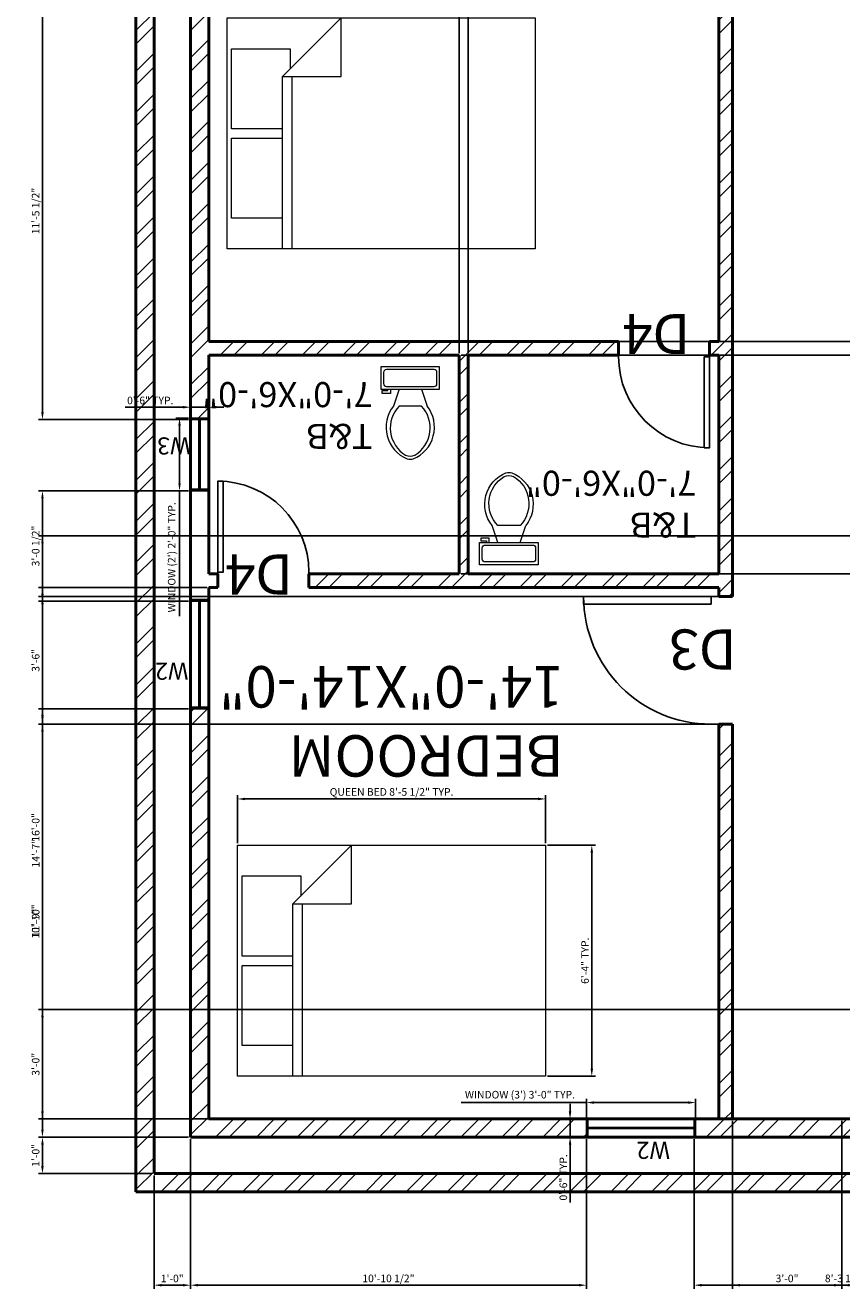
# Model space of a CAD drawing. Units: inches. Extents: x 244 to 2800, y 1060 to 1700.
# Tile 3 of 13: x 819 to 1088, y 1060 to 1477. Entities that reach past the tile are written whole.
import ezdxf

# ---------------------------------------------------------------- set-up
doc = ezdxf.new("R2010")
doc.units = ezdxf.units.IN
for name, color, linetype, lineweight in [('A-ANNO-DIMS', 2, 'Continuous', 18), ('A-ANNO-TEXT', 1, 'Continuous', 18), ('A-DOOR', 5, 'Continuous', 25), ('A-FURN', 9, 'Continuous', 18), ('A-GLAZ', 3, 'Continuous', 25), ('A-WALL', 7, 'Continuous', 50), ('A-WALL-PATT', 8, 'Continuous', 13)]:
    doc.layers.add(name, color=color, linetype=linetype, lineweight=lineweight)
doc.styles.get("Standard").update_dxf_attribs({"font": 'arial.ttf'})
doc.dimstyles.new('ISO-25', dxfattribs={"dimtxt": 2.5, "dimasz": 2.5, "dimexe": 1.25, "dimexo": 0.625, "dimtad": 1, "dimlunit": 4, "dimtxsty": 'Standard', "dimcen": 2.5, "dimadec": 0, "dimazin": 0, "dimtfac": 1, "dimtmove": 0, "dimatfit": 3, "dimfxl": 1, "dimarcsym": 0})

# ---------------------------------------------------------------- blocks, each defined once
blk = doc.blocks.new('*U2')
for p, q in [((0, 0), (0, -5)), ((30, 0), (30, -5))]:
    blk.add_line(p, q)
blk.add_lwpolyline([(0, 0), (0, 30), (1.75, 30), (1.75, 0)], close=True)
blk.add_arc((0, 0), 30, 0, 90)
blk = doc.blocks.new('Toilet - top')
for p, q in [((9.5, -6), (9.5, -2)), ((-10, -8.5), (-8, -8.5)), ((-10, -9.5), (-10, -8.5)), ((-8, -8.5), (-8, -8)), ((-7, -8), (-7, -9.5)), ((-4, -8), (-6, -14)), ((4, -8), (6, -14)), ((-7, -9.5), (-10, -9.5)), ((4, -14), (-4, -14))]:
    blk.add_line(p, q)
blk.add_lwpolyline([(10.5, -8), (10.5, 0), (-10.5, 0), (-10.5, -8)], close=True)
for points in [[(-9.5, -2), (-9.5, -6)], [(8.5, -1), (-8.5, -1)], [(-8.5, -7), (8.5, -7)]]:
    blk.add_lwpolyline(points)
for centre, radius, start, end in [((-8.62, -1.88), 0.884, 81.8699, 188.1301), ((8.62, -1.88), 0.884, 351.8699, 98.1301), ((-8.62, -6.12), 0.884, 171.8699, 278.1301), ((8.62, -6.12), 0.884, 261.8699, 8.1301), ((3.52, -21.58), 12.17, 141.4691, 247.9714), ((4.2, -21.82), 11.33, 136.3677, 238.9468), ((-3.52, -21.58), 12.17, 292.0284, 38.5307), ((-4.2, -21.82), 11.33, 301.053, 43.6321), ((0, -27.88), 4, 245.7318, 294.2682), ((0, -29), 4, 254.8605, 285.1395)]:
    blk.add_arc(centre, radius, start, end)
blk = doc.blocks.new('Bed - Queen')
for p, q in [((0, -80.00003), (0, 0)), ((0, 0), (59.99999, 0)), ((59.99999, 0), (59.99999, -80.00003)), ((7.99999, -1.2), (28.79998, -1.2)), ((7.99999, -14.4), (7.99999, -1.2)), ((28.79998, -1.2), (28.79998, -14.4)), ((31.19999, -1.2), (51.99999, -1.2)), ((31.19999, -14.4), (31.19999, -1.2)), ((51.99999, -1.2), (51.99999, -16.4)), ((0, -14.4), (44.8, -14.4)), ((59.99999, -29.6), (44.8, -14.4)), ((44.8, -14.4), (44.8, -29.6)), ((51.99999, -16.4), (46.79936, -16.4)), ((44.8, -16.8), (0, -16.8)), ((44.8, -29.6), (59.99999, -29.6)), ((59.99999, -80.00003), (0, -80.00003))]:
    blk.add_line(p, q)
blk = doc.blocks.new('WIN-36')
for p, q in [((0, 0), (0, 6)), ((0, 6), (35.94, 6)), ((35.94, 6), (35.94, 0)), ((35.94, 0), (0, 0))]:
    blk.add_line(p, q)
blk = doc.blocks.new('WIN-24')
for p, q in [((0, 0), (0, 23.94)), ((0, 23.94), (6, 23.94)), ((6, 23.94), (6, 0)), ((6, 0), (0, 0))]:
    blk.add_line(p, q)
blk = doc.blocks.new('*D54')
at = {"layer": 'A-ANNO-DIMS', "color": 0, "lineweight": -2, "transparency": 16777216}
for p, q in [((1004.16, 1122.38), (962.87, 1122.38)), ((1004.16, 1117.61), (1004.16, 1123.63)), ((1037.6, 1122.38), (1006.66, 1122.38)), ((1040.1, 1117.61), (1040.1, 1123.63))]:
    blk.add_line(p, q, dxfattribs=at)
at = {"layer": 'A-ANNO-DIMS', "color": 0, "transparency": 16777216}
for points in [[(1006.66, 1122.79), (1006.66, 1121.96), (1004.16, 1122.38)], [(1037.6, 1122.79), (1037.6, 1121.96), (1040.1, 1122.38)]]:
    blk.add_solid(points, dxfattribs=at)
at = {"layer": 'Defpoints', "color": 0, "transparency": 16777216}
for p in [(1004.16, 1122.38), (1004.16, 1116.99), (1040.1, 1116.99)]:
    blk.add_point(p, dxfattribs=at)
at = {"layer": 'A-ANNO-DIMS', "color": 0, "transparency": 16777216, "insert": (982.26, 1124.64), "char_height": 2.5, "attachment_point": 5}
blk.add_mtext('WINDOW (3\') 3\'-0" TYP.', dxfattribs=at)
blk = doc.blocks.new('*D55')
at = {"layer": 'A-ANNO-DIMS', "color": 0, "lineweight": -2, "transparency": 16777216}
for p, q in [((998.77, 1119.49), (998.77, 1121.99)), ((1003.53, 1116.99), (997.52, 1116.99)), ((998.77, 1116.99), (998.77, 1110.99)), ((1003.53, 1110.99), (997.52, 1110.99)), ((998.77, 1108.49), (998.77, 1089.5))]:
    blk.add_line(p, q, dxfattribs=at)
at = {"layer": 'A-ANNO-DIMS', "color": 0, "transparency": 16777216}
for points in [[(998.35, 1119.49), (999.18, 1119.49), (998.77, 1116.99)], [(998.35, 1108.49), (999.18, 1108.49), (998.77, 1110.99)]]:
    blk.add_solid(points, dxfattribs=at)
at = {"layer": 'Defpoints', "color": 0, "transparency": 16777216}
for p in [(1004.16, 1116.99), (998.77, 1110.99), (1004.16, 1110.99)]:
    blk.add_point(p, dxfattribs=at)
at = {"layer": 'A-ANNO-DIMS', "color": 0, "transparency": 16777216, "insert": (996.87, 1097.74), "char_height": 2.5, "attachment_point": 5, "rotation": 90}
blk.add_mtext('0\'-6" TYP.', dxfattribs=at)
blk = doc.blocks.new('*D56')
at = {"layer": 'A-ANNO-DIMS', "color": 0, "lineweight": -2, "transparency": 16777216}
for p, q in [((873.11, 1347.76), (868.89, 1347.76)), ((870.14, 1345.26), (870.14, 1326.32)), ((873.11, 1323.82), (868.89, 1323.82)), ((870.14, 1323.82), (870.14, 1282.53))]:
    blk.add_line(p, q, dxfattribs=at)
at = {"layer": 'A-ANNO-DIMS', "color": 0, "transparency": 16777216}
for points in [[(869.73, 1345.26), (870.56, 1345.26), (870.14, 1347.76)], [(869.73, 1326.32), (870.56, 1326.32), (870.14, 1323.82)]]:
    blk.add_solid(points, dxfattribs=at)
at = {"layer": 'Defpoints', "color": 0, "transparency": 16777216}
for p in [(873.74, 1347.76), (870.14, 1323.82), (873.74, 1323.82)]:
    blk.add_point(p, dxfattribs=at)
at = {"layer": 'A-ANNO-DIMS', "color": 0, "transparency": 16777216, "insert": (867.88, 1301.92), "char_height": 2.5, "attachment_point": 5, "rotation": 90}
blk.add_mtext('WINDOW (2\') 2\'-0" TYP.', dxfattribs=at)
blk = doc.blocks.new('*D57')
at = {"layer": 'A-ANNO-DIMS', "color": 0, "lineweight": -2, "transparency": 16777216}
for p, q in [((871.24, 1351.35), (852.25, 1351.35)), ((873.74, 1348.39), (873.74, 1352.6)), ((879.74, 1351.35), (873.74, 1351.35)), ((879.74, 1348.39), (879.74, 1352.6)), ((882.24, 1351.35), (884.74, 1351.35))]:
    blk.add_line(p, q, dxfattribs=at)
at = {"layer": 'A-ANNO-DIMS', "color": 0, "transparency": 16777216}
for points in [[(871.24, 1351.77), (871.24, 1350.94), (873.74, 1351.35)], [(882.24, 1351.77), (882.24, 1350.94), (879.74, 1351.35)]]:
    blk.add_solid(points, dxfattribs=at)
at = {"layer": 'Defpoints', "color": 0, "transparency": 16777216}
for p in [(873.74, 1351.35), (873.74, 1347.76), (879.74, 1347.76)]:
    blk.add_point(p, dxfattribs=at)
at = {"layer": 'A-ANNO-DIMS', "color": 0, "transparency": 16777216, "insert": (860.49, 1353.25), "char_height": 2.5, "attachment_point": 5}
blk.add_mtext('0\'-6" TYP.', dxfattribs=at)
blk = doc.blocks.new('*D62')
at = {"layer": 'A-ANNO-DIMS', "color": 0, "lineweight": -2, "transparency": 16777216}
for p, q in [((889.25, 1207.75), (889.25, 1223.6)), ((988.21, 1222.35), (891.75, 1222.35)), ((990.71, 1207.75), (990.71, 1223.6))]:
    blk.add_line(p, q, dxfattribs=at)
at = {"layer": 'A-ANNO-DIMS', "color": 0, "transparency": 16777216}
for points in [[(891.75, 1222.77), (891.75, 1221.93), (889.25, 1222.35)], [(988.21, 1222.77), (988.21, 1221.93), (990.71, 1222.35)]]:
    blk.add_solid(points, dxfattribs=at)
at = {"layer": 'Defpoints', "color": 0, "transparency": 16777216}
for p in [(889.25, 1222.35), (889.25, 1207.13), (990.71, 1207.13)]:
    blk.add_point(p, dxfattribs=at)
at = {"layer": 'A-ANNO-DIMS', "color": 0, "transparency": 16777216, "insert": (939.98, 1224.34), "char_height": 2.5, "attachment_point": 5}
blk.add_mtext('QUEEN BED 8\'-5 1/2" TYP.', dxfattribs=at)
blk = doc.blocks.new('*D63')
at = {"layer": 'A-ANNO-DIMS', "color": 0, "lineweight": -2, "transparency": 16777216}
for p, q in [((991.33, 1207.13), (1007.17, 1207.13)), ((1005.92, 1133.54), (1005.92, 1204.63)), ((991.33, 1131.04), (1007.17, 1131.04))]:
    blk.add_line(p, q, dxfattribs=at)
at = {"layer": 'A-ANNO-DIMS', "color": 0, "transparency": 16777216}
for points in [[(1005.51, 1204.63), (1006.34, 1204.63), (1005.92, 1207.13)], [(1005.51, 1133.54), (1006.34, 1133.54), (1005.92, 1131.04)]]:
    blk.add_solid(points, dxfattribs=at)
at = {"layer": 'Defpoints', "color": 0, "transparency": 16777216}
for p in [(990.71, 1207.13), (1005.92, 1207.13), (990.71, 1131.04)]:
    blk.add_point(p, dxfattribs=at)
at = {"layer": 'A-ANNO-DIMS', "color": 0, "transparency": 16777216, "insert": (1004.02, 1169.08), "char_height": 2.5, "attachment_point": 5, "rotation": 90}
blk.add_mtext('6\'-4" TYP.', dxfattribs=at)
blk = doc.blocks.new('*D111')
at = {"layer": 'A-ANNO-DIMS', "color": 0, "lineweight": -2, "transparency": 16777216}
for p, q in [((873.74, 1110.36), (873.74, 1060.99)), ((861.74, 1098.36), (861.74, 1060.99)), ((864.24, 1062.24), (871.24, 1062.24))]:
    blk.add_line(p, q, dxfattribs=at)
at = {"layer": 'A-ANNO-DIMS', "color": 0, "transparency": 16777216}
for points in [[(864.24, 1062.65), (864.24, 1061.82), (861.74, 1062.24)], [(871.24, 1062.65), (871.24, 1061.82), (873.74, 1062.24)]]:
    blk.add_solid(points, dxfattribs=at)
at = {"layer": 'Defpoints', "color": 0, "transparency": 16777216}
for p in [(873.74, 1110.99), (861.74, 1098.99), (873.74, 1062.24)]:
    blk.add_point(p, dxfattribs=at)
at = {"layer": 'A-ANNO-DIMS', "color": 0, "transparency": 16777216, "insert": (867.74, 1064.14), "char_height": 2.5, "attachment_point": 5}
blk.add_mtext('1\'-0"', dxfattribs=at)
blk = doc.blocks.new('*D112')
at = {"layer": 'A-ANNO-DIMS', "color": 0, "lineweight": -2, "transparency": 16777216}
for p, q in [((873.11, 1110.99), (823.74, 1110.99)), ((824.99, 1101.49), (824.99, 1108.49)), ((861.11, 1098.99), (823.74, 1098.99))]:
    blk.add_line(p, q, dxfattribs=at)
at = {"layer": 'A-ANNO-DIMS', "color": 0, "transparency": 16777216}
for points in [[(824.57, 1108.49), (825.4, 1108.49), (824.99, 1110.99)], [(824.57, 1101.49), (825.4, 1101.49), (824.99, 1098.99)]]:
    blk.add_solid(points, dxfattribs=at)
at = {"layer": 'Defpoints', "color": 0, "transparency": 16777216}
for p in [(824.99, 1110.99), (873.74, 1110.99), (861.74, 1098.99)]:
    blk.add_point(p, dxfattribs=at)
at = {"layer": 'A-ANNO-DIMS', "color": 0, "transparency": 16777216, "insert": (823.08, 1104.99), "char_height": 2.5, "attachment_point": 5, "rotation": 90}
blk.add_mtext('1\'-0"', dxfattribs=at)
blk = doc.blocks.new('*D118')
at = {"layer": 'A-ANNO-DIMS', "color": 0, "lineweight": -2, "transparency": 16777216}
for p, q in [((873.11, 1252.04), (823.74, 1252.04)), ((824.99, 1113.49), (824.99, 1249.54)), ((873.11, 1110.99), (823.74, 1110.99))]:
    blk.add_line(p, q, dxfattribs=at)
at = {"layer": 'A-ANNO-DIMS', "color": 0, "transparency": 16777216}
for points in [[(824.57, 1249.54), (825.4, 1249.54), (824.99, 1252.04)], [(824.57, 1113.49), (825.4, 1113.49), (824.99, 1110.99)]]:
    blk.add_solid(points, dxfattribs=at)
at = {"layer": 'Defpoints', "color": 0, "transparency": 16777216}
for p in [(824.99, 1252.04), (873.74, 1252.04), (873.74, 1110.99)]:
    blk.add_point(p, dxfattribs=at)
at = {"layer": 'A-ANNO-DIMS', "color": 0, "transparency": 16777216, "insert": (823.08, 1181.51), "char_height": 2.5, "attachment_point": 5, "rotation": 90}
blk.add_mtext('11\'-9"', dxfattribs=at)
blk = doc.blocks.new('*D119')
at = {"layer": 'A-ANNO-DIMS', "color": 0, "lineweight": -2, "transparency": 16777216}
for p, q in [((873.11, 1323.82), (823.74, 1323.82)), ((824.99, 1289.98), (824.99, 1321.32)), ((873.11, 1287.48), (823.74, 1287.48))]:
    blk.add_line(p, q, dxfattribs=at)
at = {"layer": 'A-ANNO-DIMS', "color": 0, "transparency": 16777216}
for points in [[(824.57, 1321.32), (825.4, 1321.32), (824.99, 1323.82)], [(824.57, 1289.98), (825.4, 1289.98), (824.99, 1287.48)]]:
    blk.add_solid(points, dxfattribs=at)
at = {"layer": 'Defpoints', "color": 0, "transparency": 16777216}
for p in [(824.99, 1323.82), (873.74, 1323.82), (873.74, 1287.48)]:
    blk.add_point(p, dxfattribs=at)
at = {"layer": 'A-ANNO-DIMS', "color": 0, "transparency": 16777216, "insert": (823.07, 1305.65), "char_height": 2.5, "attachment_point": 5, "rotation": 90}
blk.add_mtext('3\'-0 1/2"', dxfattribs=at)
blk = doc.blocks.new('*D120')
at = {"layer": 'A-ANNO-DIMS', "color": 0, "lineweight": -2, "transparency": 16777216}
for p, q in [((873.11, 1484.64), (823.74, 1484.64)), ((824.99, 1349.76), (824.99, 1482.14)), ((873.11, 1347.26), (823.74, 1347.26))]:
    blk.add_line(p, q, dxfattribs=at)
at = {"layer": 'A-ANNO-DIMS', "color": 0, "transparency": 16777216}
for points in [[(824.57, 1482.14), (825.4, 1482.14), (824.99, 1484.64)], [(824.57, 1349.76), (825.4, 1349.76), (824.99, 1347.26)]]:
    blk.add_solid(points, dxfattribs=at)
at = {"layer": 'Defpoints', "color": 0, "transparency": 16777216}
for p in [(824.99, 1484.64), (873.74, 1484.64), (873.74, 1347.26)]:
    blk.add_point(p, dxfattribs=at)
at = {"layer": 'A-ANNO-DIMS', "color": 0, "transparency": 16777216, "insert": (823.07, 1415.95), "char_height": 2.5, "attachment_point": 5, "rotation": 90}
blk.add_mtext('11\'-5 1/2"', dxfattribs=at)
blk = doc.blocks.new('*D123')
at = {"layer": 'A-ANNO-DIMS', "color": 0, "lineweight": -2, "transparency": 16777216}
for p, q in [((879.11, 1291.99), (823.74, 1291.99)), ((824.99, 1119.49), (824.99, 1289.49)), ((879.11, 1116.99), (823.74, 1116.99))]:
    blk.add_line(p, q, dxfattribs=at)
at = {"layer": 'A-ANNO-DIMS', "color": 0, "transparency": 16777216}
for points in [[(824.57, 1289.49), (825.4, 1289.49), (824.99, 1291.99)], [(824.57, 1119.49), (825.4, 1119.49), (824.99, 1116.99)]]:
    blk.add_solid(points, dxfattribs=at)
at = {"layer": 'Defpoints', "color": 0, "transparency": 16777216}
for p in [(824.99, 1291.99), (879.74, 1291.99), (879.74, 1116.99)]:
    blk.add_point(p, dxfattribs=at)
at = {"layer": 'A-ANNO-DIMS', "color": 0, "transparency": 16777216, "insert": (823.11, 1204.49), "char_height": 2.5, "attachment_point": 5, "rotation": 90}
blk.add_mtext('14\'-7"', dxfattribs=at)
blk = doc.blocks.new('*D124')
at = {"layer": 'A-ANNO-DIMS', "color": 0, "lineweight": -2, "transparency": 16777216}
for p, q in [((962.86, 1368.49), (1367.74, 1368.49)), ((1366.49, 1298.99), (1366.49, 1365.99)), ((962.86, 1296.49), (1367.74, 1296.49))]:
    blk.add_line(p, q, dxfattribs=at)
at = {"layer": 'A-ANNO-DIMS', "color": 0, "transparency": 16777216}
for points in [[(1366.07, 1365.99), (1366.9, 1365.99), (1366.49, 1368.49)], [(1366.07, 1298.99), (1366.9, 1298.99), (1366.49, 1296.49)]]:
    blk.add_solid(points, dxfattribs=at)
at = {"layer": 'Defpoints', "color": 0, "transparency": 16777216}
for p in [(962.24, 1368.49), (1366.49, 1368.49), (962.24, 1296.49)]:
    blk.add_point(p, dxfattribs=at)
at = {"layer": 'A-ANNO-DIMS', "color": 0, "transparency": 16777216, "insert": (1364.58, 1332.49), "char_height": 2.5, "attachment_point": 5, "rotation": 90}
blk.add_mtext('6\'-0"', dxfattribs=at)
blk = doc.blocks.new('*D125')
at = {"layer": 'A-ANNO-DIMS', "color": 0, "lineweight": -2, "transparency": 16777216}
for p, q in [((880.36, 1545.99), (1367.74, 1545.99)), ((1366.49, 1375.49), (1366.49, 1543.49)), ((880.36, 1372.99), (1367.74, 1372.99))]:
    blk.add_line(p, q, dxfattribs=at)
at = {"layer": 'A-ANNO-DIMS', "color": 0, "transparency": 16777216}
for points in [[(1366.07, 1543.49), (1366.9, 1543.49), (1366.49, 1545.99)], [(1366.07, 1375.49), (1366.9, 1375.49), (1366.49, 1372.99)]]:
    blk.add_solid(points, dxfattribs=at)
at = {"layer": 'Defpoints', "color": 0, "transparency": 16777216}
for p in [(879.74, 1545.99), (1366.49, 1545.99), (879.74, 1372.99)]:
    blk.add_point(p, dxfattribs=at)
at = {"layer": 'A-ANNO-DIMS', "color": 0, "transparency": 16777216, "insert": (1364.58, 1459.49), "char_height": 2.5, "attachment_point": 5, "rotation": 90}
blk.add_mtext('14\'-5"', dxfattribs=at)
blk = doc.blocks.new('*D126')
at = {"layer": 'A-ANNO-DIMS', "color": 0, "lineweight": -2, "transparency": 16777216}
for p, q in [((879.74, 1373.61), (879.74, 1664.99)), ((882.24, 1663.74), (959.74, 1663.74)), ((962.24, 1369.11), (962.24, 1664.99))]:
    blk.add_line(p, q, dxfattribs=at)
at = {"layer": 'A-ANNO-DIMS', "color": 0, "transparency": 16777216}
for points in [[(882.24, 1664.15), (882.24, 1663.32), (879.74, 1663.74)], [(959.74, 1664.15), (959.74, 1663.32), (962.24, 1663.74)]]:
    blk.add_solid(points, dxfattribs=at)
at = {"layer": 'Defpoints', "color": 0, "transparency": 16777216}
for p in [(962.24, 1663.74), (879.74, 1372.99), (962.24, 1368.49)]:
    blk.add_point(p, dxfattribs=at)
at = {"layer": 'A-ANNO-DIMS', "color": 0, "transparency": 16777216, "insert": (920.99, 1665.65), "char_height": 2.5, "attachment_point": 5}
blk.add_mtext('6\'-10 1/2"', dxfattribs=at)
blk = doc.blocks.new('*D127')
at = {"layer": 'A-ANNO-DIMS', "color": 0, "lineweight": -2, "transparency": 16777216}
for p, q in [((965.24, 1369.11), (965.24, 1664.99)), ((967.74, 1663.74), (1045.24, 1663.74)), ((1047.74, 1373.61), (1047.74, 1664.99))]:
    blk.add_line(p, q, dxfattribs=at)
at = {"layer": 'A-ANNO-DIMS', "color": 0, "transparency": 16777216}
for points in [[(967.74, 1664.15), (967.74, 1663.32), (965.24, 1663.74)], [(1045.24, 1664.15), (1045.24, 1663.32), (1047.74, 1663.74)]]:
    blk.add_solid(points, dxfattribs=at)
at = {"layer": 'Defpoints', "color": 0, "transparency": 16777216}
for p in [(1047.74, 1663.74), (1047.74, 1372.99), (965.24, 1368.49)]:
    blk.add_point(p, dxfattribs=at)
at = {"layer": 'A-ANNO-DIMS', "color": 0, "transparency": 16777216, "insert": (1006.49, 1665.65), "char_height": 2.5, "attachment_point": 5}
blk.add_mtext('6\'-10 1/2"', dxfattribs=at)
blk = doc.blocks.new('*D128')
at = {"layer": 'A-ANNO-DIMS', "color": 0, "lineweight": -2, "transparency": 16777216}
for p, q in [((873.74, 1110.36), (873.74, 1060.99)), ((1004.16, 1110.36), (1004.16, 1060.99)), ((876.24, 1062.24), (1001.66, 1062.24))]:
    blk.add_line(p, q, dxfattribs=at)
at = {"layer": 'A-ANNO-DIMS', "color": 0, "transparency": 16777216}
for points in [[(876.24, 1062.65), (876.24, 1061.82), (873.74, 1062.24)], [(1001.66, 1062.65), (1001.66, 1061.82), (1004.16, 1062.24)]]:
    blk.add_solid(points, dxfattribs=at)
at = {"layer": 'Defpoints', "color": 0, "transparency": 16777216}
for p in [(873.74, 1110.99), (1004.16, 1110.99), (1004.16, 1062.24)]:
    blk.add_point(p, dxfattribs=at)
at = {"layer": 'A-ANNO-DIMS', "color": 0, "transparency": 16777216, "insert": (938.95, 1064.15), "char_height": 2.5, "attachment_point": 5}
blk.add_mtext('10\'-10 1/2"', dxfattribs=at)
blk = doc.blocks.new('*D129')
at = {"layer": 'A-ANNO-DIMS', "color": 0, "lineweight": -2, "transparency": 16777216}
for p, q in [((1039.6, 1110.36), (1039.6, 1060.99)), ((1139.24, 1110.36), (1139.24, 1060.99)), ((1042.1, 1062.24), (1136.74, 1062.24))]:
    blk.add_line(p, q, dxfattribs=at)
at = {"layer": 'A-ANNO-DIMS', "color": 0, "transparency": 16777216}
for points in [[(1042.1, 1062.65), (1042.1, 1061.82), (1039.6, 1062.24)], [(1136.74, 1062.65), (1136.74, 1061.82), (1139.24, 1062.24)]]:
    blk.add_solid(points, dxfattribs=at)
at = {"layer": 'Defpoints', "color": 0, "transparency": 16777216}
for p in [(1039.6, 1110.99), (1139.24, 1110.99), (1139.24, 1062.24)]:
    blk.add_point(p, dxfattribs=at)
at = {"layer": 'A-ANNO-DIMS', "color": 0, "transparency": 16777216, "insert": (1089.42, 1064.15), "char_height": 2.5, "attachment_point": 5}
blk.add_mtext('8\'-3 1/2"', dxfattribs=at)
blk = doc.blocks.new('*D131')
at = {"layer": 'A-ANNO-DIMS', "color": 0, "lineweight": -2, "transparency": 16777216}
for p, q in [((1052.24, 1116.36), (1052.24, 1060.99)), ((1088.24, 1116.36), (1088.24, 1060.99)), ((1054.74, 1062.24), (1085.74, 1062.24))]:
    blk.add_line(p, q, dxfattribs=at)
at = {"layer": 'A-ANNO-DIMS', "color": 0, "transparency": 16777216}
for points in [[(1054.74, 1062.65), (1054.74, 1061.82), (1052.24, 1062.24)], [(1085.74, 1062.65), (1085.74, 1061.82), (1088.24, 1062.24)]]:
    blk.add_solid(points, dxfattribs=at)
at = {"layer": 'Defpoints', "color": 0, "transparency": 16777216}
for p in [(1052.24, 1116.99), (1088.24, 1116.99), (1088.24, 1062.24)]:
    blk.add_point(p, dxfattribs=at)
at = {"layer": 'A-ANNO-DIMS', "color": 0, "transparency": 16777216, "insert": (1070.24, 1064.14), "char_height": 2.5, "attachment_point": 5}
blk.add_mtext('3\'-0"', dxfattribs=at)
blk = doc.blocks.new('*D132')
at = {"layer": 'A-ANNO-DIMS', "color": 0, "lineweight": -2, "transparency": 16777216}
for p, q in [((1088.24, 1116.36), (1088.24, 1060.99)), ((1124.24, 1116.36), (1124.24, 1060.99)), ((1090.74, 1062.24), (1121.74, 1062.24))]:
    blk.add_line(p, q, dxfattribs=at)
at = {"layer": 'A-ANNO-DIMS', "color": 0, "transparency": 16777216}
for points in [[(1090.74, 1062.65), (1090.74, 1061.82), (1088.24, 1062.24)], [(1121.74, 1062.65), (1121.74, 1061.82), (1124.24, 1062.24)]]:
    blk.add_solid(points, dxfattribs=at)
at = {"layer": 'Defpoints', "color": 0, "transparency": 16777216}
for p in [(1088.24, 1116.99), (1124.24, 1116.99), (1124.24, 1062.24)]:
    blk.add_point(p, dxfattribs=at)
at = {"layer": 'A-ANNO-DIMS', "color": 0, "transparency": 16777216, "insert": (1106.24, 1064.14), "char_height": 2.5, "attachment_point": 5}
blk.add_mtext('3\'-0"', dxfattribs=at)
blk = doc.blocks.new('*D133')
at = {"layer": 'A-ANNO-DIMS', "color": 0, "lineweight": -2, "transparency": 16777216}
for p, q in [((1123.61, 1152.99), (823.74, 1152.99)), ((824.99, 1119.49), (824.99, 1150.49)), ((1123.61, 1116.99), (823.74, 1116.99))]:
    blk.add_line(p, q, dxfattribs=at)
at = {"layer": 'A-ANNO-DIMS', "color": 0, "transparency": 16777216}
for points in [[(824.57, 1150.49), (825.4, 1150.49), (824.99, 1152.99)], [(824.57, 1119.49), (825.4, 1119.49), (824.99, 1116.99)]]:
    blk.add_solid(points, dxfattribs=at)
at = {"layer": 'Defpoints', "color": 0, "transparency": 16777216}
for p in [(824.99, 1152.99), (1124.24, 1152.99), (1124.24, 1116.99)]:
    blk.add_point(p, dxfattribs=at)
at = {"layer": 'A-ANNO-DIMS', "color": 0, "transparency": 16777216, "insert": (823.08, 1134.99), "char_height": 2.5, "attachment_point": 5, "rotation": 90}
blk.add_mtext('3\'-0"', dxfattribs=at)
blk = doc.blocks.new('*D134')
at = {"layer": 'A-ANNO-DIMS', "color": 0, "lineweight": -2, "transparency": 16777216}
for p, q in [((1239.11, 1308.99), (823.74, 1308.99)), ((824.99, 1119.49), (824.99, 1306.49)), ((1239.11, 1116.99), (823.74, 1116.99))]:
    blk.add_line(p, q, dxfattribs=at)
at = {"layer": 'A-ANNO-DIMS', "color": 0, "transparency": 16777216}
for points in [[(824.57, 1306.49), (825.4, 1306.49), (824.99, 1308.99)], [(824.57, 1119.49), (825.4, 1119.49), (824.99, 1116.99)]]:
    blk.add_solid(points, dxfattribs=at)
at = {"layer": 'Defpoints', "color": 0, "transparency": 16777216}
for p in [(824.99, 1308.99), (1239.74, 1308.99), (1239.74, 1116.99)]:
    blk.add_point(p, dxfattribs=at)
at = {"layer": 'A-ANNO-DIMS', "color": 0, "transparency": 16777216, "insert": (823.08, 1212.99), "char_height": 2.5, "attachment_point": 5, "rotation": 90}
blk.add_mtext('16\'-0"', dxfattribs=at)
blk = doc.blocks.new('*D136')
at = {"layer": 'A-ANNO-DIMS', "color": 0, "lineweight": -2, "transparency": 16777216}
for p, q in [((1047.11, 1246.99), (823.74, 1246.99)), ((824.99, 1119.49), (824.99, 1244.49)), ((1047.11, 1116.99), (823.74, 1116.99))]:
    blk.add_line(p, q, dxfattribs=at)
at = {"layer": 'A-ANNO-DIMS', "color": 0, "transparency": 16777216}
for points in [[(824.57, 1244.49), (825.4, 1244.49), (824.99, 1246.99)], [(824.57, 1119.49), (825.4, 1119.49), (824.99, 1116.99)]]:
    blk.add_solid(points, dxfattribs=at)
at = {"layer": 'Defpoints', "color": 0, "transparency": 16777216}
for p in [(824.99, 1246.99), (1047.74, 1246.99), (1047.74, 1116.99)]:
    blk.add_point(p, dxfattribs=at)
at = {"layer": 'A-ANNO-DIMS', "color": 0, "transparency": 16777216, "insert": (823.08, 1181.99), "char_height": 2.5, "attachment_point": 5, "rotation": 90}
blk.add_mtext('10\'-10"', dxfattribs=at)
blk = doc.blocks.new('*D137')
at = {"layer": 'A-ANNO-DIMS', "color": 0, "lineweight": -2, "transparency": 16777216}
for p, q in [((1047.11, 1288.99), (823.74, 1288.99)), ((824.99, 1249.49), (824.99, 1286.49)), ((1047.11, 1246.99), (823.74, 1246.99))]:
    blk.add_line(p, q, dxfattribs=at)
at = {"layer": 'A-ANNO-DIMS', "color": 0, "transparency": 16777216}
for points in [[(824.57, 1286.49), (825.4, 1286.49), (824.99, 1288.99)], [(824.57, 1249.49), (825.4, 1249.49), (824.99, 1246.99)]]:
    blk.add_solid(points, dxfattribs=at)
at = {"layer": 'Defpoints', "color": 0, "transparency": 16777216}
for p in [(824.99, 1288.99), (1047.74, 1288.99), (1047.74, 1246.99)]:
    blk.add_point(p, dxfattribs=at)
at = {"layer": 'A-ANNO-DIMS', "color": 0, "transparency": 16777216, "insert": (823.08, 1267.99), "char_height": 2.5, "attachment_point": 5, "rotation": 90}
blk.add_mtext('3\'-6"', dxfattribs=at)
blk = doc.blocks.new('*D147')
at = {"layer": 'A-ANNO-DIMS', "color": 0, "lineweight": -2, "transparency": 16777216}
for p, q in [((1052.24, 1491.26), (1052.24, 1664.99)), ((1054.74, 1663.74), (1237.24, 1663.74)), ((1239.74, 1473.26), (1239.74, 1664.99))]:
    blk.add_line(p, q, dxfattribs=at)
at = {"layer": 'A-ANNO-DIMS', "color": 0, "transparency": 16777216}
for points in [[(1054.74, 1664.15), (1054.74, 1663.32), (1052.24, 1663.74)], [(1237.24, 1664.15), (1237.24, 1663.32), (1239.74, 1663.74)]]:
    blk.add_solid(points, dxfattribs=at)
at = {"layer": 'Defpoints', "color": 0, "transparency": 16777216}
for p in [(1239.74, 1663.74), (1052.24, 1490.64), (1239.74, 1472.64)]:
    blk.add_point(p, dxfattribs=at)
at = {"layer": 'A-ANNO-DIMS', "color": 0, "transparency": 16777216, "insert": (1145.99, 1665.65), "char_height": 2.5, "attachment_point": 5}
blk.add_mtext('15\'-7 1/2"', dxfattribs=at)

msp = doc.modelspace()

# ---------------------------------------------------------------- hatches: boundary and pattern name
at = {"layer": 'A-WALL-PATT'}
h = msp.add_hatch(dxfattribs=at)
h.set_pattern_fill('ANSI32', color=256)
h.paths.add_polyline_path([(1335.736, 1632.986), (855.736, 1632.986), (855.736, 1092.986), (1335.736, 1092.986)])
h.paths.add_polyline_path([(1329.736, 1626.986), (1329.736, 1098.986), (1245.736, 1098.986), (861.736, 1098.986), (861.736, 1626.986)], flags=16)
h.paths.add_polyline_path([(1245.736, 1551.986), (1245.736, 1532.64), (1239.736, 1532.64), (1239.736, 1545.986), (1137.736, 1545.986), (1137.736, 1551.986)], flags=0)
h.paths.add_polyline_path([(1196.984, 1551.986), (1196.984, 1545.986), (1161.039, 1545.986), (1161.039, 1551.986)], flags=0)
h.paths.add_polyline_path([(1196.484, 1548.786), (1161.539, 1548.786), (1161.539, 1549.186), (1196.484, 1549.186)], flags=0)
h.paths.add_polyline_path([(1245.736, 1472.64), (1245.736, 1242.986), (1281.736, 1242.986), (1281.736, 1134.986), (1293.736, 1134.986), (1293.736, 1242.986), (1329.736, 1242.986), (1329.736, 1134.986), (1245.736, 1134.986), (1245.736, 1110.986), (1139.236, 1110.986), (873.736, 1110.986), (873.736, 1484.64), (879.736, 1484.64), (879.736, 1372.986), (1014.736, 1372.986), (1014.736, 1368.486), (965.236, 1368.486), (965.236, 1296.486), (1047.736, 1296.486), (1047.736, 1368.486), (1044.736, 1368.486), (1044.736, 1372.986), (1047.736, 1372.986), (1047.736, 1490.64), (1052.236, 1490.64), (1052.236, 1288.986), (1047.736, 1288.986), (1047.736, 1291.986), (912.736, 1291.986), (912.736, 1296.486), (962.236, 1296.486), (962.236, 1368.486), (879.736, 1368.486), (879.736, 1296.486), (882.736, 1296.486), (882.736, 1291.986), (879.736, 1291.986), (879.736, 1116.986), (1047.736, 1116.986), (1047.736, 1246.986), (1052.236, 1246.986), (1052.236, 1116.986), (1088.236, 1116.986), (1088.236, 1152.986), (1088.236, 1313.486), (1095.736, 1313.486), (1095.736, 1308.986), (1092.736, 1308.986), (1092.736, 1157.486), (1128.736, 1157.486), (1128.736, 1116.986), (1139.236, 1116.986), (1175.181, 1116.986), (1239.736, 1116.986), (1239.736, 1308.986), (1137.736, 1308.986), (1137.736, 1313.486), (1239.736, 1313.486), (1239.736, 1472.64)], flags=0)
h.paths.add_polyline_path([(1245.736, 1462.542), (1245.736, 1414.597), (1239.736, 1414.597), (1239.736, 1462.542)], flags=0)
h.paths.add_polyline_path([(1242.936, 1462.042), (1242.936, 1415.097), (1242.536, 1415.097), (1242.536, 1462.042)], flags=0)
h.paths.add_polyline_path([(1095.736, 1551.986), (1095.736, 1545.986), (1052.236, 1545.986), (1052.236, 1532.64), (1047.736, 1532.64), (1047.736, 1545.986), (879.736, 1545.986), (879.736, 1532.64), (873.736, 1532.64), (873.736, 1551.986), (865.04, 1551.986), (865.04, 1623.986), (949.04, 1623.986), (949.04, 1551.986)], flags=0)
h.paths.add_polyline_path([(1020.681, 1551.986), (1020.681, 1545.986), (984.736, 1545.986), (984.736, 1551.986)], flags=0)
h.paths.add_polyline_path([(1020.181, 1548.786), (985.236, 1548.786), (985.236, 1549.186), (1020.181, 1549.186)], flags=0)
h.paths.add_polyline_path([(879.736, 1347.762), (879.736, 1323.817), (873.736, 1323.817), (873.736, 1347.762)], flags=0)
h.paths.add_polyline_path([(876.936, 1347.262), (876.936, 1324.317), (876.536, 1324.317), (876.536, 1347.262)], flags=0)
h.paths.add_polyline_path([(1124.236, 1152.986), (1124.236, 1116.986), (1088.236, 1116.986), (1088.236, 1152.986)], flags=0)
h.paths.add_polyline_path([(879.736, 1287.983), (879.736, 1252.038), (873.736, 1252.038), (873.736, 1287.983)], flags=0)
h.paths.add_polyline_path([(876.936, 1287.483), (876.936, 1252.538), (876.536, 1252.538), (876.536, 1287.483)], flags=0)
h.paths.add_polyline_path([(1175.181, 1116.986), (1175.181, 1110.986), (1139.236, 1110.986), (1139.236, 1114.186), (1174.681, 1114.186), (1174.681, 1116.986)], flags=0)
h.paths.add_polyline_path([(1040.103, 1116.986), (1040.103, 1110.986), (1004.158, 1110.986), (1004.158, 1116.986)], flags=0)
h.paths.add_polyline_path([(1039.603, 1113.786), (1004.658, 1113.786), (1004.658, 1114.186), (1039.603, 1114.186)], flags=0)
h.paths.add_polyline_path([(1164.972, 1113.308), (1150.368, 1113.308), (1150.368, 1101.713), (1164.972, 1101.713)], flags=8)
h.paths.add_polyline_path([(1033.179, 1112.552), (1018.576, 1112.552), (1018.576, 1100.958), (1033.179, 1100.958)], flags=8)
h.paths.add_polyline_path([(874.571, 1270.316), (859.967, 1270.316), (859.967, 1258.722), (874.571, 1258.722)], flags=24)
h.paths.add_polyline_path([(1011.225, 1564.465), (996.622, 1564.465), (996.622, 1552.871), (1011.225, 1552.871)], flags=8)
h.paths.add_polyline_path([(1187.63, 1564.482), (1173.026, 1564.482), (1173.026, 1552.887), (1187.63, 1552.887)], flags=8)
h.paths.add_polyline_path([(1259.132, 1444.47), (1244.529, 1444.47), (1244.529, 1432.875), (1259.132, 1432.875)], flags=8)
h.paths.add_polyline_path([(875.239, 1344.511), (860.635, 1344.511), (860.635, 1332.916), (875.239, 1332.916)], flags=24)
h.paths.add_polyline_path([(892.18, 1510.489), (862.03, 1510.489), (862.03, 1483.307), (892.18, 1483.307)], flags=8)
h.paths.add_polyline_path([(912.199, 1310.068), (882.049, 1310.068), (882.049, 1282.887), (912.199, 1282.887)], flags=8)
h.paths.add_polyline_path([(1043.03, 1389.229), (1012.88, 1389.229), (1012.88, 1362.047), (1043.03, 1362.047)], flags=8)
h.paths.add_polyline_path([(1058.3, 1285.41), (1028.149, 1285.41), (1028.149, 1258.229), (1058.3, 1258.229)], flags=8)
h.paths.add_polyline_path([(1129.051, 1325.331), (1098.901, 1325.331), (1098.901, 1298.15), (1129.051, 1298.15)], flags=8)
h.paths.add_polyline_path([(1063.761, 1526.078), (1033.611, 1526.078), (1033.611, 1498.897), (1063.761, 1498.897)], flags=8)
h.paths.add_polyline_path([(1130.374, 1573.756), (1100.224, 1573.756), (1100.224, 1546.575), (1130.374, 1546.575)], flags=8)
h.paths.add_polyline_path([(1275.672, 1516.103), (1245.522, 1516.103), (1245.522, 1488.922), (1275.672, 1488.922)], flags=8)
h.paths.add_polyline_path([(979.613, 1573.477), (979.613, 1615.869), (957.159, 1615.869), (957.159, 1573.477)], flags=8)
h.paths.add_polyline_path([(1311.481, 1266.003), (1254.484, 1266.003), (1254.484, 1252.05), (1311.481, 1252.05)], flags=8)
h.paths.add_polyline_path([(1159.757, 1266.713), (1159.757, 1153.038), (1197.594, 1153.038), (1197.594, 1266.713)], flags=8)
h.paths.add_polyline_path([(1139.055, 1456.095), (1139.055, 1323.863), (1184.409, 1323.863), (1184.409, 1456.095)], flags=8)
h.paths.add_polyline_path([(936.318, 1364.302), (878.595, 1364.302), (878.595, 1333.511), (936.318, 1333.511)], flags=8)
h.paths.add_polyline_path([(1042.961, 1335.109), (985.238, 1335.109), (985.238, 1304.318), (1042.961, 1304.318)], flags=8)
h.paths.add_polyline_path([(1002.135, 1273.839), (885.452, 1273.839), (885.452, 1222.91), (1002.135, 1222.91)], flags=8)
h.paths.add_polyline_path([(1009.771, 1532.646), (893.088, 1532.646), (893.088, 1481.717), (1009.771, 1481.717)], flags=8)
h = msp.add_hatch(dxfattribs=at)
h.set_pattern_fill('ANSI32', color=256)
h.paths.add_polyline_path([(1052.236, 1490.64), (1047.736, 1490.64), (1047.736, 1372.986), (1044.736, 1372.986), (1044.736, 1368.486), (1047.736, 1368.486), (1047.736, 1296.486), (965.236, 1296.486), (965.236, 1368.486), (1014.736, 1368.486), (1014.736, 1372.986), (879.736, 1372.986), (879.736, 1484.64), (877.736, 1484.64), (873.736, 1484.64), (873.736, 1347.762), (879.736, 1347.762), (879.736, 1368.486), (962.236, 1368.486), (962.236, 1296.486), (912.736, 1296.486), (912.736, 1291.986), (915.736, 1291.986), (1047.736, 1291.986), (1047.736, 1288.986), (1052.236, 1288.986)])
h = msp.add_hatch(dxfattribs=at)
h.set_pattern_fill('ANSI32', color=256)
h.paths.add_polyline_path([(1004.158, 1116.986), (879.736, 1116.986), (879.736, 1252.038), (873.736, 1252.038), (873.736, 1110.986), (1004.158, 1110.986)])
h = msp.add_hatch(dxfattribs=at)
h.set_pattern_fill('ANSI32', color=256)
h.paths.add_polyline_path([(1052.236, 1246.986), (1047.736, 1246.986), (1047.736, 1116.986), (1052.236, 1116.986)])
h = msp.add_hatch(dxfattribs=at)
h.set_pattern_fill('ANSI32', color=256)
h.paths.add_polyline_path([(1139.236, 1116.986), (1128.736, 1116.986), (1040.103, 1116.986), (1040.103, 1110.986), (1139.236, 1110.986)])

# ---------------------------------------------------------------- linework, layer by layer
at = {"layer": 'A-GLAZ'}
for p, q in [((873.736, 1347.262), (879.736, 1347.262)), ((876.536, 1347.262), (876.536, 1324.317)), ((876.936, 1347.262), (876.936, 1324.317)), ((879.736, 1324.317), (873.736, 1324.317)), ((873.736, 1287.483), (879.736, 1287.483)), ((876.536, 1287.483), (876.536, 1252.538)), ((876.936, 1287.483), (876.936, 1252.538)), ((879.736, 1252.538), (873.736, 1252.538)), ((1004.658, 1110.986), (1004.658, 1116.986)), ((1039.603, 1116.986), (1039.603, 1110.986)), ((1039.603, 1114.186), (1004.658, 1114.186)), ((1039.603, 1113.786), (1004.658, 1113.786))]:
    msp.add_line(p, q, dxfattribs=at)
at = {"layer": 'A-WALL'}
for p, q in [((855.736, 1632.986), (855.736, 1092.986)), ((861.736, 1626.986), (861.736, 1098.986)), ((1047.736, 1490.64), (1047.736, 1372.986)), ((1052.236, 1490.64), (1052.236, 1288.986)), ((873.736, 1484.64), (873.736, 1110.986)), ((879.736, 1484.64), (879.736, 1372.986)), ((879.736, 1372.986), (1014.736, 1372.986)), ((1014.736, 1368.486), (1014.736, 1372.986)), ((1044.736, 1372.986), (1047.736, 1372.986)), ((1047.736, 1372.986), (1044.736, 1372.986)), ((1044.736, 1372.986), (1044.736, 1368.486)), ((879.736, 1368.486), (879.736, 1296.486)), ((879.736, 1368.486), (962.236, 1368.486)), ((962.236, 1368.486), (962.236, 1296.486)), ((965.236, 1368.486), (965.236, 1296.486)), ((965.236, 1368.486), (1014.736, 1368.486)), ((1044.736, 1368.486), (1047.736, 1368.486)), ((1047.736, 1368.486), (1047.736, 1296.486)), ((879.736, 1296.486), (882.736, 1296.486)), ((882.736, 1291.986), (882.736, 1296.486)), ((912.736, 1296.486), (962.236, 1296.486)), ((912.736, 1296.486), (912.736, 1291.986)), ((965.236, 1296.486), (1047.736, 1296.486)), ((879.736, 1291.986), (879.736, 1116.986)), ((879.736, 1291.986), (882.736, 1291.986)), ((879.736, 1291.986), (882.736, 1291.986)), ((879.736, 1291.986), (882.736, 1291.986)), ((912.736, 1291.986), (1047.736, 1291.986)), ((912.736, 1291.986), (915.736, 1291.986)), ((1047.736, 1291.986), (1047.736, 1288.986)), ((1047.736, 1291.986), (1047.736, 1288.986)), ((1047.736, 1288.986), (1052.236, 1288.986)), ((1047.736, 1246.986), (1047.736, 1116.986)), ((1052.236, 1246.986), (1047.736, 1246.986)), ((1052.236, 1246.986), (1052.236, 1116.986)), ((879.736, 1116.986), (1139.236, 1116.986)), ((873.736, 1110.986), (1139.236, 1110.986)), ((861.736, 1098.986), (1329.736, 1098.986)), ((855.736, 1092.986), (1335.736, 1092.986))]:
    msp.add_line(p, q, dxfattribs=at)

# ---------------------------------------------------------------- block references
at = {"layer": 'A-DOOR', "rotation": 180}
msp.add_blockref('*U2', (1044.736, 1367.986), dxfattribs=at)
at = {"layer": 'A-DOOR'}
msp.add_blockref('*U2', (882.736, 1296.986), dxfattribs=at)
at = {"layer": 'A-DOOR', "xscale": -1.399999999999999, "yscale": 1.399999999999999, "zscale": 1.399999999999999, "rotation": 90}
msp.add_blockref('*U2', (1045.236, 1288.986), dxfattribs=at)
at = {"layer": 'A-FURN'}
for name, p, xscale, yscale, zscale, rotation in [('Bed - Queen', (885.782, 1403.45), 1.268227082860182, 1.268227082860182, 1.268227082860182, 90), ('Toilet - top', (978.628, 1299.47), -0.9221880059424842, 0.9221880059424842, 0.9221880059424842, 180), ('Bed - Queen', (889.248, 1131.036), 1.268227082860182, 1.268227082860182, 1.268227082860182, 90)]:
    msp.add_blockref(name, p, dxfattribs=dict(at, xscale=xscale, yscale=yscale, zscale=zscale, rotation=rotation))
at = {"layer": 'A-FURN', "xscale": 0.9221880059424842, "yscale": 0.9221880059424842, "zscale": 0.9221880059424842}
msp.add_blockref('Toilet - top', (946.123, 1364.643), dxfattribs=at)
at = {"layer": 'A-GLAZ'}
for name, p, rotation in [('WIN-24', (879.736, 1347.761), 180), ('WIN-36', (873.736, 1287.983), 270.0000000000006), ('WIN-36', (1040.103, 1116.986), 180)]:
    msp.add_blockref(name, p, dxfattribs=dict(at, rotation=rotation))

# ---------------------------------------------------------------- texts
at = {"layer": 'A-ANNO-TEXT', "attachment_point": 1, "rotation": 180}
for s, width, gutter_width, insert, char_height in [('D4', 20.58737, 65.951, (1038.311, 1368.836), 13.1902), ('T&B\\P7\'-0"X6\'-0"', 2.77063, 41.258, (933.709, 1337.617), 8.25169), ('W3', 2.91536, 28.132, (873.736, 1335.789), 5.6265), ('T&B\\P7\'-0"X6\'-0"', 2.77063, 41.258, (1040.352, 1308.424), 8.25169), ('D4', 20.58737, 65.951, (907.48, 1289.675), 13.1902), ('D3', 20.58737, 65.951, (1053.58, 1264.964), 13.1902), ('W2', 2.91536, 28.132, (873.068, 1261.594), 5.6265), ('BEDROOM\\P14\'-0"X14\'-0"', 25.27039, 68.243, (996.647, 1229.692), 13.64851), ('W2', 2.91536, 28.132, (1031.677, 1103.831), 5.6265)]:
    msp.add_mtext_dynamic_manual_height_columns(s, width=width, gutter_width=gutter_width, heights=[0], dxfattribs=dict(at, insert=insert, char_height=char_height))

# ---------------------------------------------------------------- dimensions: what is measured, and where the dimension line sits
at = {"layer": 'A-ANNO-DIMS'}
for base, p1, p2, picture, middle in [((962.236, 1663.736), (879.736, 1372.986), (962.236, 1368.486), '*D126', (920.986, 1665.654)), ((1047.736, 1663.736), (965.236, 1368.486), (1047.736, 1372.986), '*D127', (1006.486, 1665.654)), ((1239.736, 1663.736), (1052.236, 1490.64), (1239.736, 1472.64), '*D147', (1145.986, 1665.654)), ((1088.236, 1062.236), (1052.236, 1116.986), (1088.236, 1116.986), '*D131', (1070.236, 1064.138)), ((1124.236, 1062.236), (1088.236, 1116.986), (1124.236, 1116.986), '*D132', (1106.236, 1064.138)), ((873.736, 1062.236), (861.736, 1098.986), (873.736, 1110.986), '*D111', (867.736, 1064.138)), ((1004.158, 1062.236), (873.736, 1110.986), (1004.158, 1110.986), '*D128', (938.947, 1064.154)), ((1139.236, 1062.236), (1039.603, 1110.986), (1139.236, 1110.986), '*D129', (1089.42, 1064.155))]:
    dim = msp.add_linear_dim(base=base, p1=p1, p2=p2, dimstyle='ISO-25', override={"dimdec": 1, "dimlfac": 1, "dimrnd": 0, "dimzin": 1, "dimdsep": 46, "dimlunit": 4, "dimfrac": 2}, dxfattribs=at)
    dim.commit()
    dim.dimension.update_dxf_attribs({"geometry": picture, "text_midpoint": middle})
for base, p1, p2, picture, middle in [((1366.486, 1545.986), (879.736, 1372.986), (879.736, 1545.986), '*D125', (1364.585, 1459.486)), ((824.986, 1484.64), (873.736, 1347.262), (873.736, 1484.64), '*D120', (823.068, 1415.951)), ((1366.486, 1368.486), (962.236, 1296.486), (962.236, 1368.486), '*D124', (1364.585, 1332.486)), ((824.986, 1323.817), (873.736, 1287.483), (873.736, 1323.817), '*D119', (823.068, 1305.65)), ((824.986, 1308.986), (1239.736, 1116.986), (1239.736, 1308.986), '*D134', (823.085, 1212.986)), ((824.986, 1291.986), (879.736, 1116.986), (879.736, 1291.986), '*D123', (823.106, 1204.486)), ((824.986, 1288.986), (1047.736, 1246.986), (1047.736, 1288.986), '*D137', (823.084, 1267.986)), ((824.986, 1252.038), (873.736, 1110.986), (873.736, 1252.038), '*D118', (823.085, 1181.512)), ((824.986, 1246.986), (1047.736, 1116.986), (1047.736, 1246.986), '*D136', (823.085, 1181.986)), ((824.986, 1152.986), (1124.236, 1116.986), (1124.236, 1152.986), '*D133', (823.084, 1134.986)), ((824.986, 1110.986), (861.736, 1098.986), (873.736, 1110.986), '*D112', (823.085, 1104.986))]:
    dim = msp.add_linear_dim(base=base, p1=p1, p2=p2, angle=90, dimstyle='ISO-25', override={"dimdec": 1, "dimlfac": 1, "dimrnd": 0, "dimzin": 1, "dimdsep": 46, "dimlunit": 4, "dimfrac": 2}, dxfattribs=at)
    dim.commit()
    dim.dimension.update_dxf_attribs({"geometry": picture, "text_midpoint": middle})
for base, p1, p2, angle, text, picture, middle in [((873.736, 1351.353), (879.736, 1347.762), (873.736, 1347.762), 180, '<> TYP.', '*D57', (860.492, 1353.255)), ((870.144, 1323.817), (873.736, 1347.762), (873.736, 1323.817), 270, "WINDOW (2') <> TYP.", '*D56', (867.88, 1301.921)), ((889.248, 1222.349), (990.706, 1207.13), (889.248, 1207.13), 180, 'QUEEN BED <> TYP.', '*D62', (939.977, 1224.343)), ((1005.925, 1207.13), (990.706, 1131.036), (990.706, 1207.13), 90, '<> TYP.', '*D63', (1004.023, 1169.083)), ((1004.158, 1122.378), (1040.103, 1116.986), (1004.158, 1116.986), 180, "WINDOW (3') <> TYP.", '*D54', (982.263, 1124.643)), ((998.766, 1110.986), (1004.158, 1116.986), (1004.158, 1110.986), 270, '<> TYP.', '*D55', (996.865, 1097.742))]:
    dim = msp.add_linear_dim(base=base, p1=p1, p2=p2, angle=angle, text=text, dimstyle='ISO-25', override={"dimdec": 1, "dimrnd": 0, "dimzin": 1, "dimlunit": 4, "dimfrac": 2}, dxfattribs=at)
    dim.commit()
    dim.dimension.update_dxf_attribs({"geometry": picture, "text_midpoint": middle})

doc.saveas('drawing.dxf')
